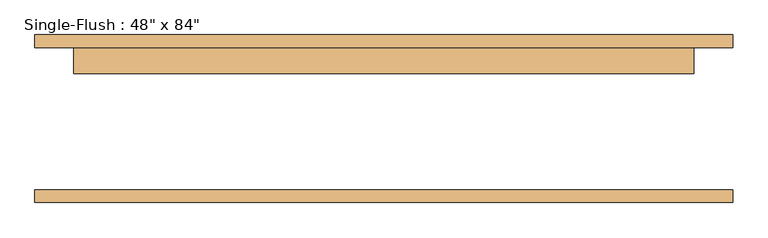
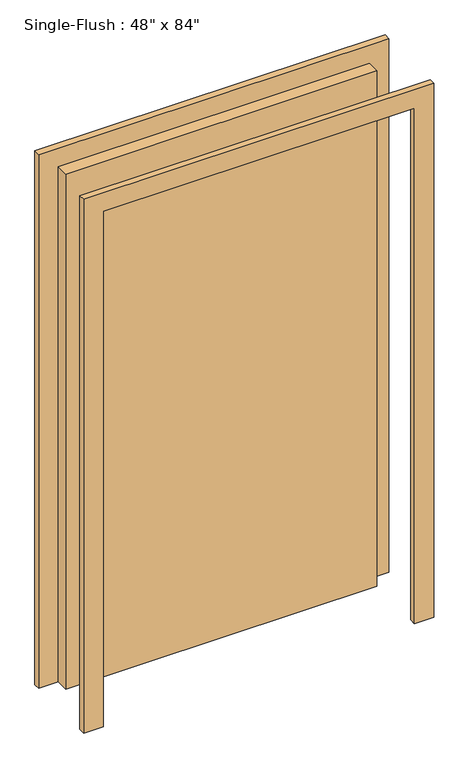
"""IFC4 building model written with IfcOpenShell, lengths in millimetres: door geometry."""

from ifc_helpers import new_model, si_unit, frame, origin, origin_with_axes, place, context, project, spatial, polyline, outline, extrude, source, transform, mapped, element, save


def door_21b9160b(model_context):
    return source(origin(), model_context, "Body", "SweptSolid", [
        extrude(outline(polyline([(2209.8, -685.8), (0.0, -685.8), (0.0, -609.6), (2133.6, -609.6), (2133.6, 609.6), (0.0, 609.6), (0.0, 685.8), (2209.8, 685.8), (2209.8, -685.8)])), frame((0.0, 139.7, 0.0), z_axis=(0.0, 1.0, 0.0), x_axis=(0.0, 0.0, 1.0)), (0.0, 0.0, 1.0), 25.4),
        extrude(outline(polyline([(2209.8, 685.8), (2209.8, -685.8), (0.0, -685.8), (0.0, -609.6), (2133.6, -609.6), (2133.6, 609.6), (0.0, 609.6), (0.0, 685.8), (2209.8, 685.8)])), frame((0.0, -165.1, 0.0), z_axis=(0.0, 1.0, 0.0), x_axis=(0.0, 0.0, 1.0)), (0.0, 0.0, 1.0), 25.4),
        extrude(outline(polyline([(609.6, 88.9), (-609.6, 88.9), (-609.6, 139.7), (609.6, 139.7), (609.6, 88.9)])), origin_with_axes(), (0.0, 0.0, 1.0), 2133.6),
    ])


if __name__ == "__main__":
    model = new_model("IFC4")
    model_context = context("Model", 3, world=origin())
    ifc_project = project(units=[si_unit("LENGTHUNIT", "METRE", prefix="MILLI")], contexts=[model_context])
    site = spatial("IfcSite", under=ifc_project)
    building = spatial("IfcBuilding", under=site)
    placement = place(None, origin())
    door_shape = door_21b9160b(model_context)
    element("IfcDoor", 1, ObjectType="Single-Flush : 48\" x 84\"", at=placement, inside=building, context=model_context, shape_type="MappedRepresentation", body=[
        mapped(door_shape, transform((0.0, 0.0, 0.0), x_axis=(1.0, 0.0, 0.0), y_axis=(0.0, 1.0, 0.0), z_axis=(0.0, 0.0, 1.0))),
    ])
    save(model, "model.ifc")

# Revit data of these elements
# Type "Single-Flush : 48\" x 84\""
#   Type Mark = "8"
#   Construction Type Id = "MDOOR"
#   Assembly Code = "C1020"
#   Analytic Construction = "Metal"
#   Thickness = 0' - 2"
#   Heat Transfer Coefficient (U) = 0.651978 BTU/(h·ft²·°F)
#   Height = 7' - 0"
#   Trim Projection Ext = 0' - 1"
#   Trim Projection Int = 0' - 1"
#   Trim Width = 0' - 3"
#   Width = 4' - 0"
#   Define Thermal Properties by = 1
#   Door Material = Door - Panel
#   Frame Material = Door - Frame
#   Visual Light Transmittance = 0
#   Solar Heat Gain Coefficient = 0
#   Function = (empty or 0)
#   Wall Closure = (empty or 0)
# Element 1 (IfcDoor, "Single-Flush : 48\" x 84\"")
#   Materials on its faces: "Door - Frame", "Door - Panel"
# Materials
#   "Door - Panel": class "Wood", colour RGB 210 159 95, transparency 0, Cost = 0
#   "Door - Frame": colour RGB 118 70 51, transparency 0, Cost = 0
